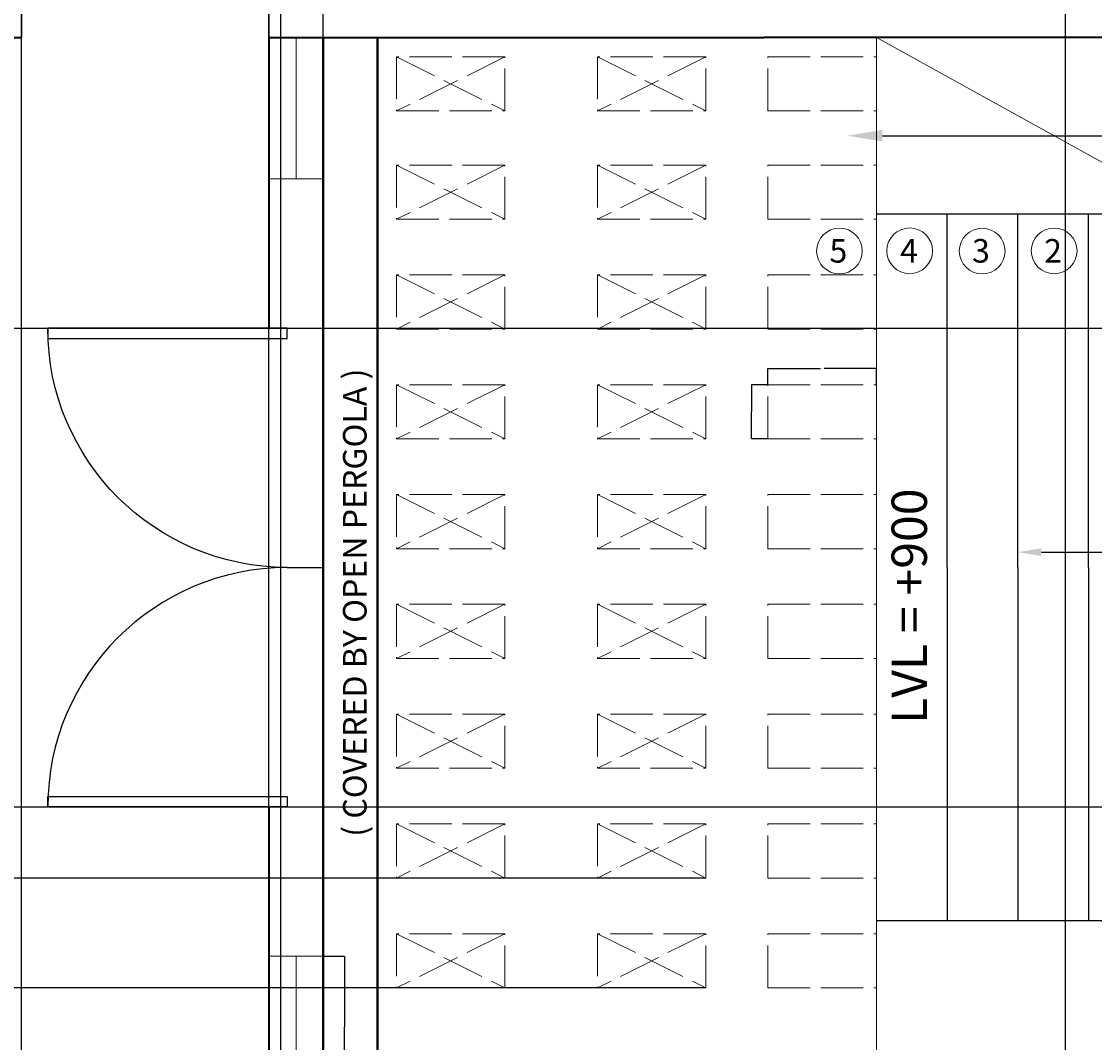
# Model space of a CAD drawing. Units: millimetres. Extents: x -8052 to 19968, y -37825 to -17505.
# Tile 5 of 10: x 5980 to 10533, y -29741 to -25407. Entities that reach past the tile are written whole.
import ezdxf
from ezdxf import colors
from ezdxf.entities.mleader import LeaderData, LeaderLine
from ezdxf.math import Vec2, Vec3

# ---------------------------------------------------------------- set-up
doc = ezdxf.new("R2010")
doc.units = ezdxf.units.MM
doc.header["$MEASUREMENT"] = 0
doc.linetypes.add('ACAD_ISO02W100', pattern=[15, 12, -3])
for name, color, linetype, lineweight in [('A-ANNO-DIMS', 2, 'Continuous', 18), ('A-ANNO-SYMB', 7, 'Continuous', 18), ('A-ANNO-TEXT', 7, 'Continuous', 18), ('A-DOOR', 3, 'Continuous', 25), ('A-FLOR', 8, 'Continuous', 18), ('A-FLOR-STRS', 7, 'Continuous', 25), ('A-GLAZ', 4, 'Continuous', 18), ('A-ROOF-OVHD', 8, 'ACAD_ISO02W100', 18), ('A-WALL', 7, 'Continuous', 35)]:
    doc.layers.add(name, color=color, linetype=linetype, lineweight=lineweight)
doc.styles.get("Standard").update_dxf_attribs({"font": 'arial.ttf'})
doc.dimstyles.get("Standard").update_dxf_attribs({"dimtxt": 1.054, "dimasz": 1.055, "dimexe": 0.18, "dimexo": 0.0625, "dimgap": 0.09, "dimtad": 0, "dimtih": 1, "dimtoh": 1, "dimdec": 4, "dimzin": 0, "dimdsep": 46, "dimtxsty": 'Standard', "dimcen": 0.09, "dimadec": 0, "dimazin": 0, "dimtfac": 1, "dimtdec": 4, "dimtofl": 0, "dimtmove": 0, "dimatfit": 3, "dimfxl": 1, "dimtolj": 1, "dimtzin": 0, "dimarcsym": 0})

# ---------------------------------------------------------------- blocks, each defined once
blk = doc.blocks.new('*U20')
for p, q in [((0, 0), (0, -6)), ((-40, 0), (-40, -6))]:
    blk.add_line(p, q)
blk.add_lwpolyline([(0, 0), (0, 40), (-1.75, 40), (-1.75, 0)], close=True)
blk.add_arc((0, 0), 40, 90, 180)
blk = doc.blocks.new('*U21')
for p, q in [((0, 0), (0, -6)), ((40, 0), (40, -6))]:
    blk.add_line(p, q)
blk.add_lwpolyline([(0, 0), (0, 40), (1.75, 40), (1.75, 0)], close=True)
blk.add_arc((0, 0), 40, 0, 90)
blk = doc.blocks.new('PERGOLA-CROSSED-MEMBER')
at = {"ltscale": 15}
for p, q in [((0, 230), (460, 0)), ((460, 230), (0, 0))]:
    blk.add_line(p, q, dxfattribs=at)
blk.add_lwpolyline([(0, 230), (460, 230), (460, 0), (0, 0)], close=True, dxfattribs=at)
blk = doc.blocks.new('PERGOLA-EDGE-MEMBER')
at = {"ltscale": 15}
for p, q in [((461.5, 230), (0, 230)), ((461.5, 230), (461.5, 0)), ((461.5, 0), (0, 0))]:
    blk.add_line(p, q, dxfattribs=at)
blk = doc.blocks.new('STAIR-SIDE-ENTRY-3000')
for p, q in [((0, 1500), (0, 3000)), ((0, 3000), (1200, 3000)), ((300, 1500), (300, 3000)), ((300, 1500), (300, 3000)), ((600, 1500), (600, 3000)), ((900, 1500), (900, 3000)), ((0, 1500), (0, 1500)), ((0, 1500), (0, 0)), ((300, 1500), (300, 0)), ((600, 1500), (600, 0)), ((900, 1500), (900, 0)), ((0, 0), (1200, 0))]:
    blk.add_line(p, q)
blk = doc.blocks.new('WIN-SIDE-600')
for p, q in [((115, 0), (115, 600)), ((0, 0), (230, 0))]:
    blk.add_line(p, q)
blk = doc.blocks.new('*D54')
at = {"layer": 'A-ANNO-DIMS', "color": 0, "lineweight": -2, "transparency": 16777216}
for p, q in [((7260, -29374.8), (7350.2, -29374.8)), ((7350, -29375.9), (7350, -29674.2)), ((7350, -29973.8), (7350, -29675.5)), ((7260, -29974.8), (7350.2, -29974.8))]:
    blk.add_line(p, q, dxfattribs=at)
at = {"layer": 'A-ANNO-DIMS', "color": 0, "lineweight": 100, "transparency": 16777216}
for points in [[(7349.8, -29375.9), (7350.2, -29375.9), (7350, -29374.8)], [(7349.8, -29973.8), (7350.2, -29973.8), (7350, -29974.8)]]:
    blk.add_solid(points, dxfattribs=at)
at = {"layer": 'Defpoints', "color": 0, "lineweight": 100, "transparency": 16777216}
for p in [(7260, -29374.8), (7260, -29974.8), (7350, -29974.8)]:
    blk.add_point(p, dxfattribs=at)
at = {"layer": 'A-ANNO-DIMS', "color": 0, "transparency": 16777216, "insert": (7350, -29674.8), "char_height": 1.054, "attachment_point": 5}
blk.add_mtext('\\A1;SIDE WINDOW 600 TYP.', dxfattribs=at)
blk = doc.blocks.new('*D82')
at = {"layer": 'A-ANNO-DIMS', "color": 0, "lineweight": -2, "transparency": 16777216}
for p, q in [((9146, -26948.9), (9146, -26879.6)), ((9147.1, -26879.8), (9368, -26879.8)), ((9606.4, -26879.8), (9385.5, -26879.8)), ((9607.5, -26948.9), (9607.5, -26879.6))]:
    blk.add_line(p, q, dxfattribs=at)
at = {"layer": 'A-ANNO-DIMS', "color": 0, "lineweight": 100, "transparency": 16777216}
for points in [[(9147.1, -26879.6), (9147.1, -26879.9), (9146, -26879.8)], [(9606.4, -26879.6), (9606.4, -26879.9), (9607.5, -26879.8)]]:
    blk.add_solid(points, dxfattribs=at)
at = {"layer": 'Defpoints', "color": 0, "lineweight": 100, "transparency": 16777216}
for p in [(9146, -26879.8), (9146, -26949), (9607.5, -26949)]:
    blk.add_point(p, dxfattribs=at)
at = {"layer": 'A-ANNO-DIMS', "color": 0, "transparency": 16777216, "insert": (9376.7, -26879.8), "char_height": 1.054, "attachment_point": 5}
blk.add_mtext('\\A1;EDGE MEMBER 461 TYP.', dxfattribs=at)
blk = doc.blocks.new('*D83')
at = {"layer": 'A-ANNO-DIMS', "color": 0, "lineweight": -2, "transparency": 16777216}
for p, q in [((9145.9, -26949), (9076.6, -26949)), ((9076.8, -26950), (9076.8, -27063.3)), ((9076.8, -27177.9), (9076.8, -27064.6)), ((9145.9, -27179), (9076.6, -27179))]:
    blk.add_line(p, q, dxfattribs=at)
at = {"layer": 'A-ANNO-DIMS', "color": 0, "lineweight": 100, "transparency": 16777216}
for points in [[(9076.6, -26950), (9077, -26950), (9076.8, -26949)], [(9076.6, -27177.9), (9077, -27177.9), (9076.8, -27179)]]:
    blk.add_solid(points, dxfattribs=at)
at = {"layer": 'Defpoints', "color": 0, "lineweight": 100, "transparency": 16777216}
for p in [(9146, -26949), (9076.8, -27179), (9146, -27179)]:
    blk.add_point(p, dxfattribs=at)
at = {"layer": 'A-ANNO-DIMS', "color": 0, "transparency": 16777216, "insert": (9076.8, -27064), "char_height": 1.054, "attachment_point": 5}
blk.add_mtext('\\A1;230 TYP.', dxfattribs=at)
blk = doc.blocks.new('*D97')
at = {"layer": 'A-ANNO-DIMS', "color": 0, "lineweight": -2, "transparency": 16777216}
for p, q in [((12090, -25474.8), (14099.7, -25474.8)), ((14099.5, -25475.9), (14099.5, -27724.2)), ((14099.5, -29973.8), (14099.5, -27725.5)), ((10410, -29974.8), (14099.7, -29974.8))]:
    blk.add_line(p, q, dxfattribs=at)
at = {"layer": 'A-ANNO-DIMS', "color": 0, "lineweight": 100, "transparency": 16777216}
for points in [[(14099.3, -25475.9), (14099.7, -25475.9), (14099.5, -25474.8)], [(14099.3, -29973.8), (14099.7, -29973.8), (14099.5, -29974.8)]]:
    blk.add_solid(points, dxfattribs=at)
at = {"layer": 'Defpoints', "color": 0, "lineweight": 100, "transparency": 16777216}
for p in [(12090, -25474.8), (10410, -29974.8), (14099.5, -29974.8)]:
    blk.add_point(p, dxfattribs=at)
at = {"layer": 'A-ANNO-DIMS', "color": 0, "transparency": 16777216, "insert": (14099.5, -27724.8), "char_height": 1.05, "attachment_point": 5}
blk.add_mtext('\\A1;4500', dxfattribs=at)
blk = doc.blocks.new('*D104')
at = {"layer": 'A-ANNO-DIMS', "color": 0, "lineweight": -2, "transparency": 16777216}
for p, q in [((5980, -35400), (5980, -17505.2)), ((5981, -17505.3), (6528.4, -17505.3)), ((7078.9, -17505.3), (6531.6, -17505.3)), ((7080, -35584.8), (7080, -17505.2))]:
    blk.add_line(p, q, dxfattribs=at)
at = {"layer": 'A-ANNO-DIMS', "color": 0, "lineweight": 100, "transparency": 16777216}
for points in [[(5981, -17505.2), (5981, -17505.5), (5980, -17505.3)], [(7078.9, -17505.2), (7078.9, -17505.5), (7080, -17505.3)]]:
    blk.add_solid(points, dxfattribs=at)
at = {"layer": 'Defpoints', "color": 0, "lineweight": 100, "transparency": 16777216}
for p in [(7080, -17505.3), (5980, -35400), (7080, -35584.8)]:
    blk.add_point(p, dxfattribs=at)
at = {"layer": 'A-ANNO-DIMS', "color": 0, "transparency": 16777216, "insert": (6530, -17505.3), "char_height": 1.05, "attachment_point": 5}
blk.add_mtext('\\A1;1100', dxfattribs=at)
blk = doc.blocks.new('*D108')
at = {"layer": 'A-ANNO-DIMS', "color": 0, "lineweight": -2, "transparency": 16777216}
for p, q in [((-330, -29974.8), (-330, -17505.2)), ((-329, -17505.3), (3348.3, -17505.3)), ((7028.9, -17505.3), (3351.6, -17505.3)), ((7030, -29974.8), (7030, -17505.2))]:
    blk.add_line(p, q, dxfattribs=at)
at = {"layer": 'A-ANNO-DIMS', "color": 0, "lineweight": 100, "transparency": 16777216}
for points in [[(-329, -17505.2), (-329, -17505.5), (-330, -17505.3)], [(7028.9, -17505.2), (7028.9, -17505.5), (7030, -17505.3)]]:
    blk.add_solid(points, dxfattribs=at)
at = {"layer": 'Defpoints', "color": 0, "lineweight": 100, "transparency": 16777216}
for p in [(7030, -17505.3), (-330, -29974.8), (7030, -29974.8)]:
    blk.add_point(p, dxfattribs=at)
at = {"layer": 'A-ANNO-DIMS', "color": 0, "transparency": 16777216, "insert": (3350, -17505.3), "char_height": 1.05, "attachment_point": 5}
blk.add_mtext('\\A1;7360', dxfattribs=at)
blk = doc.blocks.new('*D111')
at = {"layer": 'A-ANNO-DIMS', "color": 0, "lineweight": -2, "transparency": 16777216}
for p, q in [((-560, -26708.8), (14099.7, -26708.8)), ((14099.5, -26709.9), (14099.5, -27724.2)), ((14099.5, -28739.8), (14099.5, -27725.5)), ((-560, -28740.8), (14099.7, -28740.8))]:
    blk.add_line(p, q, dxfattribs=at)
at = {"layer": 'A-ANNO-DIMS', "color": 0, "lineweight": 100, "transparency": 16777216}
for points in [[(14099.3, -26709.9), (14099.7, -26709.9), (14099.5, -26708.8)], [(14099.3, -28739.8), (14099.7, -28739.8), (14099.5, -28740.8)]]:
    blk.add_solid(points, dxfattribs=at)
at = {"layer": 'Defpoints', "color": 0, "lineweight": 100, "transparency": 16777216}
for p in [(-560, -26708.8), (-560, -28740.8), (14099.5, -28740.8)]:
    blk.add_point(p, dxfattribs=at)
at = {"layer": 'A-ANNO-DIMS', "color": 0, "transparency": 16777216, "insert": (14099.5, -27724.8), "char_height": 1.05, "attachment_point": 5}
blk.add_mtext('\\A1;2032', dxfattribs=at)
blk = doc.blocks.new('*D112')
at = {"layer": 'A-ANNO-DIMS', "color": 0, "lineweight": -2, "transparency": 16777216}
for p, q in [((8883.8, -29042.9), (-8049.7, -29042.9)), ((-8049.5, -29043.9), (-8049.5, -29275.2)), ((-8049.5, -29507.8), (-8049.5, -29276.5)), ((8883.8, -29508.9), (-8049.7, -29508.9))]:
    blk.add_line(p, q, dxfattribs=at)
at = {"layer": 'A-ANNO-DIMS', "color": 0, "lineweight": 100, "transparency": 16777216}
for points in [[(-8049.7, -29043.9), (-8049.3, -29043.9), (-8049.5, -29042.9)], [(-8049.7, -29507.8), (-8049.3, -29507.8), (-8049.5, -29508.9)]]:
    blk.add_solid(points, dxfattribs=at)
at = {"layer": 'Defpoints', "color": 0, "lineweight": 100, "transparency": 16777216}
for p in [(8883.8, -29042.9), (-8049.5, -29508.9), (8883.8, -29508.9)]:
    blk.add_point(p, dxfattribs=at)
at = {"layer": 'A-ANNO-DIMS', "color": 0, "transparency": 16777216, "insert": (-8049.5, -29275.9), "char_height": 1.05, "attachment_point": 5}
blk.add_mtext('\\A1;466', dxfattribs=at)
blk = doc.blocks.new('*D123')
at = {"layer": 'A-ANNO-DIMS', "color": 0, "lineweight": -2, "transparency": 16777216}
for p, q in [((7260, -25474.8), (7260, -17505.2)), ((7261, -17505.3), (9673.3, -17505.3)), ((12088.9, -17505.3), (9676.7, -17505.3)), ((12090, -25474.8), (12090, -17505.2))]:
    blk.add_line(p, q, dxfattribs=at)
at = {"layer": 'A-ANNO-DIMS', "color": 0, "lineweight": 100, "transparency": 16777216}
for points in [[(7261, -17505.2), (7261, -17505.5), (7260, -17505.3)], [(12088.9, -17505.2), (12088.9, -17505.5), (12090, -17505.3)]]:
    blk.add_solid(points, dxfattribs=at)
at = {"layer": 'Defpoints', "color": 0, "lineweight": 100, "transparency": 16777216}
for p in [(7260, -17505.3), (7260, -25474.8), (12090, -25474.8)]:
    blk.add_point(p, dxfattribs=at)
at = {"layer": 'A-ANNO-DIMS', "color": 0, "transparency": 16777216, "insert": (9675, -17505.3), "char_height": 1.05, "attachment_point": 5}
blk.add_mtext('\\A1;4830', dxfattribs=at)
blk = doc.blocks.new('*D124')
at = {"layer": 'A-ANNO-DIMS', "color": 0, "lineweight": -2, "transparency": 16777216}
for p, q in [((7030, -29974.8), (7030, -17505.2)), ((7031, -17505.3), (8718.3, -17505.3)), ((10408.9, -17505.3), (8721.6, -17505.3)), ((10410, -29974.8), (10410, -17505.2))]:
    blk.add_line(p, q, dxfattribs=at)
at = {"layer": 'A-ANNO-DIMS', "color": 0, "lineweight": 100, "transparency": 16777216}
for points in [[(7031, -17505.2), (7031, -17505.5), (7030, -17505.3)], [(10408.9, -17505.2), (10408.9, -17505.5), (10410, -17505.3)]]:
    blk.add_solid(points, dxfattribs=at)
at = {"layer": 'Defpoints', "color": 0, "lineweight": 100, "transparency": 16777216}
for p in [(10410, -17505.3), (7030, -29974.8), (10410, -29974.8)]:
    blk.add_point(p, dxfattribs=at)
at = {"layer": 'A-ANNO-DIMS', "color": 0, "transparency": 16777216, "insert": (8720, -17505.3), "char_height": 1.05, "attachment_point": 5}
blk.add_mtext('\\A1;3380', dxfattribs=at)

msp = doc.modelspace()

# ---------------------------------------------------------------- linework, layer by layer
at = {"layer": 'A-ANNO-SYMB'}
for centre in [(9450.443, -26381.699), (9748.355, -26380.846), (10055.92, -26381.938), (10361.268, -26381.051)]:
    msp.add_circle(centre, 97, dxfattribs=at)
at = {"layer": 'A-FLOR'}
for p, q in [((9607.479, -25474.843), (9607.479, -29974.843)), ((9607.479, -25474.843), (9607.479, -29974.843)), ((11409.979, -26474.843), (9607.479, -25474.843))]:
    msp.add_line(p, q, dxfattribs=at)
at = {"layer": 'A-WALL'}
for p, q in [((5579.979, -25474.843), (5979.979, -25474.843)), ((7029.979, -25474.843), (9129.979, -25474.843)), ((7029.979, -25474.843), (7029.979, -26708.843)), ((7259.979, -29974.843), (7259.979, -25474.843)), ((7259.979, -25474.843), (7259.979, -29974.843)), ((7489.979, -29974.843), (7489.979, -25474.843)), ((7489.979, -25474.843), (7489.979, -29974.843)), ((9359.979, -25474.843), (9129.979, -25474.843)), ((11859.979, -25474.843), (9359.979, -25474.843)), ((7029.979, -28740.843), (7029.979, -29974.843))]:
    msp.add_line(p, q, dxfattribs=at)

# ---------------------------------------------------------------- block references
at = {"layer": 'A-DOOR', "xscale": 26.25, "yscale": 26.25, "zscale": 26.25}
msp.add_blockref('*U20', (7029.979, -25317.343), dxfattribs=at)
at = {"layer": 'A-DOOR', "yscale": 25.4, "zscale": 25.4}
for p, xscale, rotation in [((7107.579, -26708.843), -25.4, 90), ((7107.579, -28740.843), 25.4, 90.00000000000003)]:
    msp.add_blockref('*U21', p, dxfattribs=dict(at, xscale=xscale, rotation=rotation))
at = {"layer": 'A-FLOR-STRS', "extrusion": (0, 0, -1), "zscale": -1}
msp.add_blockref('STAIR-SIDE-ENTRY-3000', (-10807.48, -29224.843), dxfattribs=at)
at = {"layer": 'A-GLAZ'}
msp.add_blockref('WIN-SIDE-600', (7029.979, -26074.843), dxfattribs=at)
at = {"layer": 'A-GLAZ', "rotation": 180}
msp.add_blockref('WIN-SIDE-600', (7259.98, -29374.843), dxfattribs=at)
at = {"layer": 'A-ROOF-OVHD', "extrusion": (0, 0, -1), "zscale": -1}
for p in [(-8031.275, -25787.023), (-8883.837, -25787.023), (-8031.275, -26247.023), (-8883.837, -26247.023), (-8031.275, -26713), (-8883.837, -26713), (-8031.275, -27178.978), (-8883.837, -27178.978), (-8031.275, -27644.955), (-8883.837, -27644.955), (-8031.275, -28110.933), (-8883.837, -28110.933), (-8031.275, -28576.91), (-8883.837, -28576.91), (-8031.275, -29042.888), (-8883.837, -29042.888), (-8031.275, -29508.865), (-8883.837, -29508.865)]:
    msp.add_blockref('PERGOLA-CROSSED-MEMBER', p, dxfattribs=at)
at = {"layer": 'A-ROOF-OVHD', "rotation": 180}
for p in [(9607.48, -25557.023), (9607.48, -26017.023), (9607.48, -26483.001), (9607.48, -26948.978), (9607.48, -27414.956), (9607.48, -27880.933), (9607.48, -28346.911), (9607.48, -28812.888), (9607.48, -29278.866)]:
    msp.add_blockref('PERGOLA-EDGE-MEMBER', p, dxfattribs=at)

# ---------------------------------------------------------------- texts
at = {"layer": 'A-ANNO-TEXT', "char_height": 100, "attachment_point": 3}
for s, insert in [('5', (9483.595, -26330.846)), ('4', (9782.939, -26330.846)), ('3', (10088.662, -26330.846)), ('2', (10394.386, -26330.846))]:
    msp.add_mtext_dynamic_manual_height_columns(s, width=159.07556, gutter_width=1, heights=[0], dxfattribs=dict(at, insert=insert))
at = {"layer": 'A-ANNO-TEXT', "attachment_point": 7, "rotation": 90}
for s, width, insert, char_height in [('( COVERED BY OPEN PERGOLA )', 2294.41831, (7444.201, -28867.616), 100), ('LVL = +900', 1598.33979, (9821.536, -28388.9), 150)]:
    msp.add_mtext_dynamic_manual_height_columns(s, width=width, gutter_width=1, heights=[0], dxfattribs=dict(at, insert=insert, char_height=char_height))

# ---------------------------------------------------------------- dimensions: what is measured, and where the dimension line sits
at = {"layer": 'A-ANNO-DIMS'}
for base, p1, p2, picture, middle in [((7029.979, -17505.343), (-330.021, -29974.843), (7029.979, -29974.843), '*D108', (3349.979, -17505.343)), ((7079.979, -17505.343), (5979.979, -35400.039), (7079.979, -35584.843), '*D104', (6529.979, -17505.343)), ((10409.979, -17505.343), (7029.979, -29974.843), (10409.979, -29974.843), '*D124', (8719.979, -17505.343)), ((7259.979, -17505.343), (12089.979, -25474.843), (7259.979, -25474.843), '*D123', (9674.979, -17505.343))]:
    dim = msp.add_linear_dim(base=base, p1=p1, p2=p2, dimstyle='Standard', override={"dimdec": 0, "dimlfac": 1, "dimrnd": 0, "dimzin": 0, "dimdsep": 46, "dimlunit": 2}, dxfattribs=at)
    dim.commit()
    dim.dimension.update_dxf_attribs({"geometry": picture, "text_midpoint": middle})
for base, p1, p2, picture, middle in [((14099.479, -29974.843), (12089.979, -25474.843), (10409.979, -29974.843), '*D97', (14099.479, -27724.843)), ((14099.479, -28740.843), (-560.021, -26708.843), (-560.021, -28740.843), '*D111', (14099.479, -27724.843)), ((-8049.521, -29508.866), (8883.837, -29042.888), (8883.837, -29508.866), '*D112', (-8049.521, -29275.877))]:
    dim = msp.add_linear_dim(base=base, p1=p1, p2=p2, angle=90, dimstyle='Standard', override={"dimdec": 0, "dimlfac": 1, "dimrnd": 0, "dimzin": 0, "dimdsep": 46, "dimlunit": 2}, dxfattribs=at)
    dim.commit()
    dim.dimension.update_dxf_attribs({"geometry": picture, "text_midpoint": middle})
for base, p1, p2, angle, text, picture, middle in [((9146.002, -26879.756), (9607.479, -26948.978), (9146.002, -26948.978), 180, 'EDGE MEMBER <> TYP.', '*D82', (9376.741, -26879.756)), ((9076.781, -27178.978), (9146.002, -26948.978), (9146.002, -27178.978), 270, '<> TYP.', '*D83', (9076.781, -27063.978)), ((7349.979, -29974.843), (7259.979, -29374.843), (7259.979, -29974.843), 270, 'SIDE WINDOW <> TYP.', '*D54', (7349.979, -29674.843))]:
    dim = msp.add_linear_dim(base=base, p1=p1, p2=p2, angle=angle, text=text, dimstyle='Standard', override={"dimdec": 0, "dimlfac": 1, "dimrnd": 0, "dimzin": 0, "dimdsep": 46, "dimlunit": 2}, dxfattribs=at)
    dim.commit()
    dim.dimension.update_dxf_attribs({"geometry": picture, "text_midpoint": middle})

# ---------------------------------------------------------------- leaders
at = {"layer": 'A-ANNO-TEXT'}
ml = msp.add_multileader_mtext('Standard', dxfattribs=at)
ml.set_content('230 TH DW WALL', color=256)
ml.set_leader_properties()
ml.build(insert=Vec2(0, 0))
ml.multileader.update_dxf_attribs({"dogleg_length": 0.36, "arrow_head_size": 150})
ctx = ml.context
ctx.base_point, ctx.char_height, ctx.arrow_head_size, ctx.landing_gap_size, ctx.plane_origin = Vec3(10841.096, -25892.244), 100, 150, 0.09, Vec3(9482.701, -25892.244)
notes = []
notes.append((ctx, [(0, (1, 1, 0), (10840.736, -25892.244), (1, 0), 0.36, [(0, [(9482.701, -25892.244)], 0, [])])]))
ctx.mtext.insert, ctx.mtext.flow_direction = Vec3(10841.186, -25841.357), 5
ml = msp.add_multileader_mtext('Standard', dxfattribs=at)
ml.set_content('\\pxt1;UP', color=256)
ml.set_leader_properties()
ml.build(insert=Vec2(0, 0))
ml.multileader.update_dxf_attribs({"dogleg_length": 0.36, "arrow_head_size": 100})
ctx = ml.context
ctx.base_point, ctx.char_height, ctx.arrow_head_size, ctx.landing_gap_size, ctx.plane_origin = Vec3(11617.533, -27659.789), 100, 100, 0.09, Vec3(10207.479, -27659.789)
notes.append((ctx, [(0, (1, 1, 0), (11617.173, -27659.789), (1, 0), 0.36, [(0, [(10207.479, -27659.789)], 0, [])])]))
ctx.mtext.insert, ctx.mtext.width, ctx.mtext.flow_direction = Vec3(11617.623, -27608.937), 0.34019, 5
for ctx, leaders in notes:
    for number, flags, end, landing, length, lines in leaders:
        leader = LeaderData()
        leader.index, (leader.has_last_leader_line, leader.has_dogleg_vector, leader.attachment_direction) = number, flags
        leader.last_leader_point, leader.dogleg_vector, leader.dogleg_length = Vec3(end), Vec3(landing), length
        for number, points, colour, breaks in lines:
            line = LeaderLine()
            line.index, line.vertices, line.color, line.breaks = number, Vec3.list(points), colors.encode_raw_color(colour), breaks
            leader.lines.append(line)
        ctx.leaders.append(leader)

doc.saveas('drawing.dxf')
